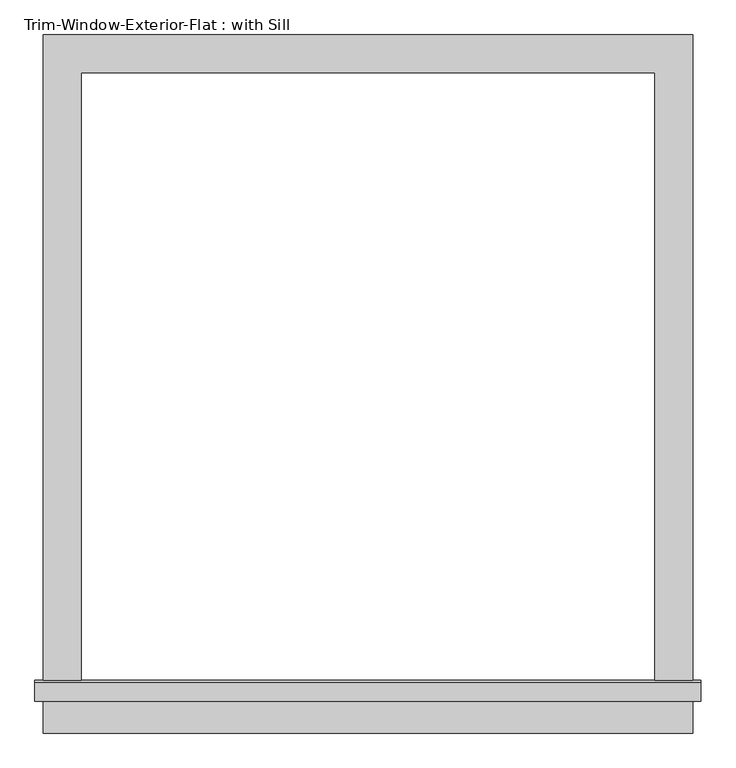
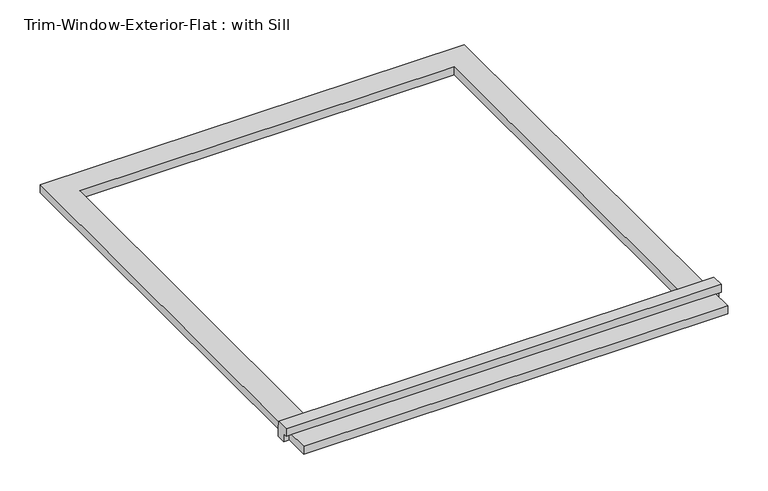
"""IFC4 building model written with IfcOpenShell, lengths in millimetres: proxy geometry, Trim-Window-Exterior-Flat : with Sill."""

from ifc_helpers import new_model, si_unit, frame, origin, origin_with_axes, place, context, project, spatial, polyline, outline, extrude, source, transform, mapped, element, save


def trim_window_exterior_flat_with_sill_41619996(model_context):
    return source(origin(), model_context, "Body", "SweptSolid", [
        extrude(outline(polyline([(488.95, -936.5823709), (488.95, -993.7323709), (-488.95, -993.7323709), (-488.95, -936.5823709), (488.95, -936.5823709)])), origin_with_axes(), (0.0, 0.0, 1.0), 19.05),
        extrude(outline(polyline([(-946.15, 38.1), (-916.8580645, 38.1), (-914.4, 19.05), (-914.4, 0.0), (-936.5823709, 0.0), (-936.5823709, 19.05), (-946.15, 19.05), (-946.15, 38.1)])), frame((-501.65, 0.0, 0.0), z_axis=(1.0, 0.0, 0.0), x_axis=(0.0, 1.0, 0.0)), (0.0, 0.0, 1.0), 1003.3),
        extrude(outline(polyline([(-488.95, 57.15), (488.95, 57.15), (488.95, -914.4), (431.8, -914.4), (431.8, 0.0), (-431.8, 0.0), (-431.8, -914.4), (-488.95, -914.4), (-488.95, 57.15)])), origin_with_axes(), (0.0, 0.0, 1.0), 19.05),
    ])


if __name__ == "__main__":
    model = new_model("IFC4")
    model_context = context("Model", 3, world=origin())
    ifc_project = project(units=[si_unit("LENGTHUNIT", "METRE", prefix="MILLI")], contexts=[model_context])
    site = spatial("IfcSite", under=ifc_project)
    building = spatial("IfcBuilding", under=site)
    placement = place(None, origin())
    trim_window_exterior_flat_with_sill_shape = trim_window_exterior_flat_with_sill_41619996(model_context)
    element("IfcBuildingElementProxy", 1, Name="Trim-Window-Exterior-Flat : with Sill", ObjectType="Trim-Window-Exterior-Flat : with Sill", at=placement, inside=building, context=model_context, shape_type="MappedRepresentation", body=[
        mapped(trim_window_exterior_flat_with_sill_shape, transform((0.0, 0.0, 0.0), x_axis=(1.0, 0.0, 0.0), y_axis=(0.0, 1.0, 0.0), z_axis=(0.0, 0.0, 1.0))),
    ])
    save(model, "model.ifc")

# Revit data of these elements
# Type "Trim-Window-Exterior-Flat : with Sill"
#   Trim Width = 0.1875 ft
#   Trim Thickness_Picture Frame = 0.104167 ft
#   Trim Thickness_with Sill = 0.0625 ft
#   Sill Thickness = 0.104167 ft
#   Opening Width [instance default] = 2 ft
#   Opening Height [instance default] = 3 ft
#   Default Elevation = 4 ft
#   Sill = yes
#   Picture Frame = no
#   Trim Material [instance default] = none
# Element 1 (IfcBuildingElementProxy, "Trim-Window-Exterior-Flat : with Sill")
#   Opening Width = 2.833333 ft
#   Trim Material = Clad - White
#   Materials on its faces: "Clad - White"
# Materials
#   "Clad - White": class "Wood", colour RGB 242 242 238, transparency 0, Cost = 0
